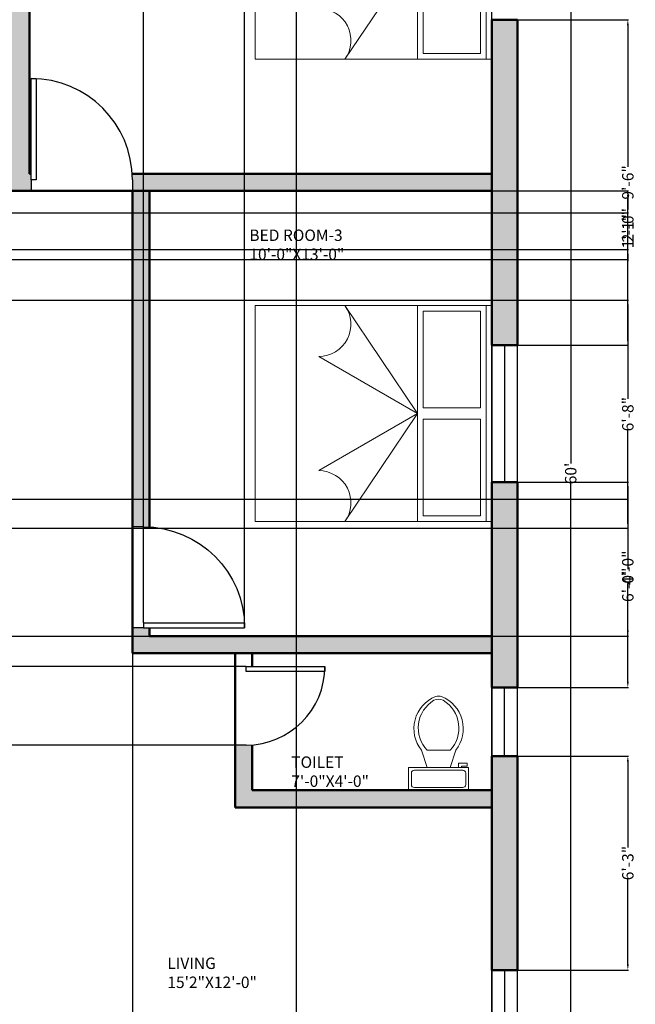
# Model space of a CAD drawing. Units: inches. Extents: x 2430 to 2930, y 1715 to 2575.
# Tile 3 of 4: x 2711 to 2927, y 1933 to 2278. Entities that reach past the tile are written whole.
import ezdxf

# ---------------------------------------------------------------- set-up
doc = ezdxf.new("R2010")
doc.units = ezdxf.units.IN
for name, color, linetype, lineweight in [('A-ANNO-DIMS', 2, 'Continuous', 18), ('A-AREA-IDEN', 130, 'Continuous', 18), ('A-FLOR-FIXT', 200, 'Continuous', 18), ('A-FURN', 200, 'Continuous', 18), ('A-WALL', 7, 'Continuous', 50), ('A-WALL-PATT', 251, 'Continuous', 13), ('DOOR', 224, 'Continuous', 25), ('win', 170, 'Continuous', 25)]:
    doc.layers.add(name, color=color, linetype=linetype, lineweight=lineweight)
doc.styles.get("Standard").update_dxf_attribs({"font": 'arial.ttf', "height": 4})
doc.dimstyles.get("Standard").update_dxf_attribs({"dimtxt": 4, "dimasz": 2, "dimexe": 0.18, "dimexo": 0.0625, "dimgap": 0.09, "dimtad": 0, "dimzin": 0, "dimdsep": 46, "dimlunit": 3, "dimtxsty": 'Standard', "dimcen": 0.09, "dimadec": 0, "dimazin": 0, "dimtfac": 1, "dimtofl": 0, "dimtmove": 0, "dimatfit": 3, "dimfxl": 1, "dimtolj": 1, "dimtzin": 0, "dimarcsym": 0})

# ---------------------------------------------------------------- blocks, each defined once
blk = doc.blocks.new('*U4')
for p, q in [((0, 0), (0, -100)), ((700, 0), (700, -100))]:
    blk.add_line(p, q)
blk.add_lwpolyline([(0, 0), (0, 700), (43.75, 700), (43.75, 0)], close=True)
blk.add_arc((0, 0), 700, 0, 90)
blk = doc.blocks.new('*U7')
for p, q in [((0, 0), (0, -100)), ((900, 0), (900, -100))]:
    blk.add_line(p, q)
blk.add_lwpolyline([(0, 0), (0, 900), (43.75, 900), (43.75, 0)], close=True)
blk.add_arc((0, 0), 900, 0, 90)
blk = doc.blocks.new('*U9')
for p, q in [((241.3, -152.4), (241.3, -50.8)), ((-254, -215.9), (-203.2, -215.9)), ((-254, -241.3), (-254, -215.9)), ((-177.8, -241.3), (-254, -241.3)), ((-203.2, -215.9), (-203.2, -203.2)), ((-177.8, -203.2), (-177.8, -241.3)), ((-101.6, -203.2), (-152.4, -355.6)), ((101.6, -203.2), (152.4, -355.6)), ((101.6, -355.6), (-101.6, -355.6))]:
    blk.add_line(p, q)
blk.add_lwpolyline([(266.7, -203.2), (266.7, 0), (-266.7, 0), (-266.7, -203.2)], close=True)
for points in [[(-241.3, -50.8), (-241.3, -152.4)], [(215.9, -25.4), (-215.9, -25.4)], [(-215.9, -177.8), (215.9, -177.8)]]:
    blk.add_lwpolyline(points)
for centre, radius, start, end in [((-219.1, -47.6), 22.5, 81.8699, 188.1301), ((219.1, -47.6), 22.5, 351.8699, 98.1301), ((-219.1, -155.6), 22.5, 171.8699, 278.1301), ((219.1, -155.6), 22.5, 261.8699, 8.1301), ((89.4, -548.1), 309.1, 141.46911, 247.97143), ((106.7, -554.2), 287.8, 136.36773, 238.94682), ((-89.4, -548.1), 309.1, 292.02843, 38.53071), ((-106.7, -554.2), 287.8, 301.05301, 43.63209), ((0, -708.1), 101.6, 245.73182, 294.26817), ((0, -736.6), 101.6, 254.86053, 285.13947)]:
    blk.add_arc(centre, radius, start, end)
blk = doc.blocks.new('NEW BED')
for p, q in [((-75.7, 82.92), (0, 82.92)), ((-75.7, 0), (-75.7, 82.92)), ((0, 82.92), (0, 0)), ((-75.7, 80.92), (0, 80.92)), ((-73.7, 78.92), (-39.85, 78.92)), ((-73.7, 58.92), (-73.7, 78.92)), ((-39.85, 58.92), (-39.85, 78.92)), ((-35.85, 78.92), (-2, 78.92)), ((-35.85, 58.92), (-35.85, 78.92)), ((-2, 78.92), (-2, 58.92)), ((-73.7, 58.92), (-39.85, 58.92)), ((-35.85, 58.92), (-2, 58.92)), ((-75.7, 56.92), (0, 56.92)), ((-37.85, 56.92), (-75.7, 31.45)), ((-37.85, 56.92), (-57.85, 22.27)), ((-37.85, 56.92), (0, 31.45)), ((-37.85, 56.92), (-17.84, 22.27)), ((0, 0), (-75.7, 0))]:
    blk.add_line(p, q)
for centre, start, end in [((-69.14, 22.27), 0, 125.5497), ((-6.56, 22.27), 54.4503, 180)]:
    blk.add_arc(centre, 11.28, start, end)
blk = doc.blocks.new('*D12')
at = {"layer": 'A-ANNO-DIMS', "color": 0, "lineweight": -2, "transparency": 16777216}
for p, q in [((2885.68, 2479.45), (2904.48, 2479.45)), ((2904.3, 2477.45), (2904.3, 2122.95)), ((2904.3, 1761.45), (2904.3, 2115.96)), ((2885.68, 1759.45), (2904.48, 1759.45))]:
    blk.add_line(p, q, dxfattribs=at)
at = {"layer": 'A-ANNO-DIMS', "color": 0, "transparency": 16777216}
for points in [[(2903.96, 2477.45), (2904.63, 2477.45), (2904.3, 2479.45)], [(2903.96, 1761.45), (2904.63, 1761.45), (2904.3, 1759.45)]]:
    blk.add_solid(points, dxfattribs=at)
at = {"layer": 'Defpoints', "color": 0, "transparency": 16777216}
for p in [(2885.62, 2479.45), (2885.62, 1759.45), (2904.3, 1759.45)]:
    blk.add_point(p, dxfattribs=at)
at = {"layer": 'A-ANNO-DIMS', "color": 0, "transparency": 16777216, "insert": (2904.3, 2119.45), "char_height": 4, "attachment_point": 5, "rotation": 90}
blk.add_mtext("\\A1;60'", dxfattribs=at)
blk = doc.blocks.new('WIN-48IN')
blk.add_line((0, 4.5), (48, 4.5))
blk.add_lwpolyline([(0, 9), (48, 9), (48, 0), (0, 0)], close=True)
blk = doc.blocks.new('WIN-24IN')
blk.add_line((24, 4.5), (0, 4.5))
blk.add_lwpolyline([(0, 9), (24, 9), (24, 0), (0, 0)], close=True)
blk = doc.blocks.new('*D25')
at = {"layer": 'A-ANNO-DIMS', "color": 0, "lineweight": -2, "transparency": 16777216}
for p, q in [((2754.56, 2067.12), (2754.56, 2569.33)), ((2756.56, 2569.15), (2760.62, 2569.15)), ((2787.99, 2569.15), (2783.93, 2569.15)), ((2789.99, 2067.12), (2789.99, 2569.33))]:
    blk.add_line(p, q, dxfattribs=at)
at = {"layer": 'A-ANNO-DIMS', "color": 0, "transparency": 16777216}
for points in [[(2756.56, 2569.49), (2756.56, 2568.82), (2754.56, 2569.15)], [(2787.99, 2569.49), (2787.99, 2568.82), (2789.99, 2569.15)]]:
    blk.add_solid(points, dxfattribs=at)
at = {"layer": 'Defpoints', "color": 0, "transparency": 16777216}
for p in [(2789.99, 2569.15), (2754.56, 2067.05), (2789.99, 2067.05)]:
    blk.add_point(p, dxfattribs=at)
at = {"layer": 'A-ANNO-DIMS', "color": 0, "transparency": 16777216, "insert": (2772.27, 2569.15), "char_height": 4, "attachment_point": 5}
blk.add_mtext('\\A1;2\'-11 1/2"', dxfattribs=at)
blk = doc.blocks.new('*D26')
at = {"layer": 'A-ANNO-DIMS', "color": 0, "lineweight": -2, "transparency": 16777216}
for p, q in [((2786.56, 2051.85), (2435.74, 2051.85)), ((2435.92, 2049.85), (2435.92, 2048.17)), ((2435.92, 2026.29), (2435.92, 2027.97)), ((2786.56, 2024.29), (2435.74, 2024.29))]:
    blk.add_line(p, q, dxfattribs=at)
at = {"layer": 'A-ANNO-DIMS', "color": 0, "transparency": 16777216}
for points in [[(2435.59, 2049.85), (2436.25, 2049.85), (2435.92, 2051.85)], [(2435.59, 2026.29), (2436.25, 2026.29), (2435.92, 2024.29)]]:
    blk.add_solid(points, dxfattribs=at)
at = {"layer": 'Defpoints', "color": 0, "transparency": 16777216}
for p in [(2435.92, 2051.85), (2786.62, 2051.85), (2786.62, 2024.29)]:
    blk.add_point(p, dxfattribs=at)
at = {"layer": 'A-ANNO-DIMS', "color": 0, "transparency": 16777216, "insert": (2435.92, 2038.07), "char_height": 4, "attachment_point": 5, "rotation": 90}
blk.add_mtext('\\A1;2\'-3 1/2"', dxfattribs=at)
blk = doc.blocks.new('*D35')
at = {"layer": 'A-ANNO-DIMS', "color": 0, "lineweight": -2, "transparency": 16777216}
for p, q in [((2885.68, 2278.45), (2924.5, 2278.45)), ((2924.32, 2276.45), (2924.32, 2226.86)), ((2924.32, 2166.45), (2924.32, 2216.05)), ((2885.68, 2164.45), (2924.5, 2164.45))]:
    blk.add_line(p, q, dxfattribs=at)
at = {"layer": 'A-ANNO-DIMS', "color": 0, "transparency": 16777216}
for points in [[(2923.99, 2276.45), (2924.65, 2276.45), (2924.32, 2278.45)], [(2923.99, 2166.45), (2924.65, 2166.45), (2924.32, 2164.45)]]:
    blk.add_solid(points, dxfattribs=at)
at = {"layer": 'Defpoints', "color": 0, "transparency": 16777216}
for p in [(2885.62, 2278.45), (2885.62, 2164.45), (2924.32, 2164.45)]:
    blk.add_point(p, dxfattribs=at)
at = {"layer": 'A-ANNO-DIMS', "color": 0, "transparency": 16777216, "insert": (2924.32, 2221.45), "char_height": 4, "attachment_point": 5, "rotation": 90}
blk.add_mtext('\\A1;9\'-6"', dxfattribs=at)
blk = doc.blocks.new('*D36')
at = {"layer": 'A-ANNO-DIMS', "color": 0, "lineweight": -2, "transparency": 16777216}
for p, q in [((2885.68, 2116.45), (2924.5, 2116.45)), ((2924.32, 2114.45), (2924.32, 2085.87)), ((2924.32, 2046.45), (2924.32, 2075.04)), ((2885.68, 2044.45), (2924.5, 2044.45))]:
    blk.add_line(p, q, dxfattribs=at)
at = {"layer": 'A-ANNO-DIMS', "color": 0, "transparency": 16777216}
for points in [[(2923.99, 2114.45), (2924.65, 2114.45), (2924.32, 2116.45)], [(2923.99, 2046.45), (2924.65, 2046.45), (2924.32, 2044.45)]]:
    blk.add_solid(points, dxfattribs=at)
at = {"layer": 'Defpoints', "color": 0, "transparency": 16777216}
for p in [(2885.62, 2116.45), (2885.62, 2044.45), (2924.32, 2044.45)]:
    blk.add_point(p, dxfattribs=at)
at = {"layer": 'A-ANNO-DIMS', "color": 0, "transparency": 16777216, "insert": (2924.32, 2080.45), "char_height": 4, "attachment_point": 5, "rotation": 90}
blk.add_mtext('\\A1;6\'-0"', dxfattribs=at)
blk = doc.blocks.new('*D37')
at = {"layer": 'A-ANNO-DIMS', "color": 0, "lineweight": -2, "transparency": 16777216}
for p, q in [((2885.68, 2020.45), (2924.5, 2020.45)), ((2924.32, 2018.45), (2924.32, 1988.37)), ((2924.32, 1947.45), (2924.32, 1977.54)), ((2885.68, 1945.45), (2924.5, 1945.45))]:
    blk.add_line(p, q, dxfattribs=at)
at = {"layer": 'A-ANNO-DIMS', "color": 0, "transparency": 16777216}
for points in [[(2923.99, 2018.45), (2924.65, 2018.45), (2924.32, 2020.45)], [(2923.99, 1947.45), (2924.65, 1947.45), (2924.32, 1945.45)]]:
    blk.add_solid(points, dxfattribs=at)
at = {"layer": 'Defpoints', "color": 0, "transparency": 16777216}
for p in [(2885.62, 2020.45), (2885.62, 1945.45), (2924.32, 1945.45)]:
    blk.add_point(p, dxfattribs=at)
at = {"layer": 'A-ANNO-DIMS', "color": 0, "transparency": 16777216, "insert": (2924.32, 1982.95), "char_height": 4, "attachment_point": 5, "rotation": 90}
blk.add_mtext('\\A1;6\'-3"', dxfattribs=at)
blk = doc.blocks.new('*D39')
at = {"layer": 'A-ANNO-DIMS', "color": 0, "lineweight": -2, "transparency": 16777216}
for p, q in [((2808.12, 1840.52), (2808.12, 2569.33)), ((2810.12, 2569.15), (2832.3, 2569.15)), ((2874.62, 2569.15), (2852.44, 2569.15)), ((2876.62, 1840.52), (2876.62, 2569.33))]:
    blk.add_line(p, q, dxfattribs=at)
at = {"layer": 'A-ANNO-DIMS', "color": 0, "transparency": 16777216}
for points in [[(2810.12, 2569.49), (2810.12, 2568.82), (2808.12, 2569.15)], [(2874.62, 2569.49), (2874.62, 2568.82), (2876.62, 2569.15)]]:
    blk.add_solid(points, dxfattribs=at)
at = {"layer": 'Defpoints', "color": 0, "transparency": 16777216}
for p in [(2876.62, 2569.15), (2808.12, 1840.45), (2876.62, 1840.45)]:
    blk.add_point(p, dxfattribs=at)
at = {"layer": 'A-ANNO-DIMS', "color": 0, "transparency": 16777216, "insert": (2842.37, 2569.15), "char_height": 4, "attachment_point": 5}
blk.add_mtext('\\A1;5\'-8 1/2"', dxfattribs=at)
blk = doc.blocks.new('*D40')
at = {"layer": 'A-ANNO-DIMS', "color": 0, "lineweight": -2, "transparency": 16777216}
for p, q in [((2630.68, 2180.15), (2924.5, 2180.15)), ((2924.32, 2178.15), (2924.32, 2145.66)), ((2924.32, 2102.32), (2924.32, 2134.82)), ((2630.68, 2100.32), (2924.5, 2100.32))]:
    blk.add_line(p, q, dxfattribs=at)
at = {"layer": 'A-ANNO-DIMS', "color": 0, "transparency": 16777216}
for points in [[(2923.99, 2178.15), (2924.65, 2178.15), (2924.32, 2180.15)], [(2923.99, 2102.32), (2924.65, 2102.32), (2924.32, 2100.32)]]:
    blk.add_solid(points, dxfattribs=at)
at = {"layer": 'Defpoints', "color": 0, "transparency": 16777216}
for p in [(2630.62, 2180.15), (2924.32, 2180.15), (2630.62, 2100.32)]:
    blk.add_point(p, dxfattribs=at)
at = {"layer": 'A-ANNO-DIMS', "color": 0, "transparency": 16777216, "insert": (2924.32, 2140.24), "char_height": 4, "attachment_point": 5, "rotation": 90}
blk.add_mtext('\\A1;6\'-8"', dxfattribs=at)
blk = doc.blocks.new('*D41')
at = {"layer": 'A-ANNO-DIMS', "color": 0, "lineweight": -2, "transparency": 16777216}
for p, q in [((2693.62, 2062.39), (2693.62, 1720.57)), ((2750.62, 2056.39), (2750.62, 1720.57)), ((2695.62, 1720.75), (2716.63, 1720.75)), ((2748.62, 1720.75), (2727.61, 1720.75))]:
    blk.add_line(p, q, dxfattribs=at)
at = {"layer": 'A-ANNO-DIMS', "color": 0, "transparency": 16777216}
for points in [[(2695.62, 1721.09), (2695.62, 1720.42), (2693.62, 1720.75)], [(2748.62, 1721.09), (2748.62, 1720.42), (2750.62, 1720.75)]]:
    blk.add_solid(points, dxfattribs=at)
at = {"layer": 'Defpoints', "color": 0, "transparency": 16777216}
for p in [(2693.62, 2062.45), (2750.62, 2056.45), (2750.62, 1720.75)]:
    blk.add_point(p, dxfattribs=at)
at = {"layer": 'A-ANNO-DIMS', "color": 0, "transparency": 16777216, "insert": (2722.12, 1720.75), "char_height": 4, "attachment_point": 5}
blk.add_mtext('\\A1;4\'-9"', dxfattribs=at)
blk = doc.blocks.new('*D50')
at = {"layer": 'A-ANNO-DIMS', "color": 0, "lineweight": -2, "transparency": 16777216}
for p, q in [((2536.91, 2110.42), (2924.5, 2110.42)), ((2924.32, 2108.42), (2924.32, 2091.92)), ((2924.32, 2064.45), (2924.32, 2080.95)), ((2534.68, 2062.45), (2924.5, 2062.45))]:
    blk.add_line(p, q, dxfattribs=at)
at = {"layer": 'A-ANNO-DIMS', "color": 0, "transparency": 16777216}
for points in [[(2923.99, 2108.42), (2924.65, 2108.42), (2924.32, 2110.42)], [(2923.99, 2064.45), (2924.65, 2064.45), (2924.32, 2062.45)]]:
    blk.add_solid(points, dxfattribs=at)
at = {"layer": 'Defpoints', "color": 0, "transparency": 16777216}
for p in [(2536.85, 2110.42), (2534.62, 2062.45), (2924.32, 2062.45)]:
    blk.add_point(p, dxfattribs=at)
at = {"layer": 'A-ANNO-DIMS', "color": 0, "transparency": 16777216, "insert": (2924.32, 2086.44), "char_height": 4, "attachment_point": 5, "rotation": 90}
blk.add_mtext('\\A1;4\'-0"', dxfattribs=at)
blk = doc.blocks.new('*D52')
at = {"layer": 'A-ANNO-DIMS', "color": 0, "lineweight": -2, "transparency": 16777216}
for p, q in [((2924.32, 2212.78), (2924.32, 2214.78)), ((2608.57, 2210.78), (2924.5, 2210.78)), ((2613.81, 2197.89), (2924.5, 2197.89)), ((2924.32, 2195.89), (2924.32, 2193.89))]:
    blk.add_line(p, q, dxfattribs=at)
at = {"layer": 'A-ANNO-DIMS', "color": 0, "transparency": 16777216}
for points in [[(2923.99, 2212.78), (2924.65, 2212.78), (2924.32, 2210.78)], [(2923.99, 2195.89), (2924.65, 2195.89), (2924.32, 2197.89)]]:
    blk.add_solid(points, dxfattribs=at)
at = {"layer": 'Defpoints', "color": 0, "transparency": 16777216}
for p in [(2608.51, 2210.78), (2924.32, 2210.78), (2613.75, 2197.89)]:
    blk.add_point(p, dxfattribs=at)
at = {"layer": 'A-ANNO-DIMS', "color": 0, "transparency": 16777216, "insert": (2924.32, 2204.34), "char_height": 4, "attachment_point": 5, "rotation": 90}
blk.add_mtext('\\A1;1\'-1"', dxfattribs=at)
blk = doc.blocks.new('*D54')
at = {"layer": 'A-ANNO-DIMS', "color": 0, "lineweight": -2, "transparency": 16777216}
for p, q in [((2624.68, 2218.45), (2924.5, 2218.45)), ((2924.32, 2216.45), (2924.32, 2211.89)), ((2924.32, 2196.45), (2924.32, 2201.01)), ((2624.68, 2194.45), (2924.5, 2194.45))]:
    blk.add_line(p, q, dxfattribs=at)
at = {"layer": 'A-ANNO-DIMS', "color": 0, "transparency": 16777216}
for points in [[(2923.99, 2216.45), (2924.65, 2216.45), (2924.32, 2218.45)], [(2923.99, 2196.45), (2924.65, 2196.45), (2924.32, 2194.45)]]:
    blk.add_solid(points, dxfattribs=at)
at = {"layer": 'Defpoints', "color": 0, "transparency": 16777216}
for p in [(2624.62, 2218.45), (2924.32, 2218.45), (2624.62, 2194.45)]:
    blk.add_point(p, dxfattribs=at)
at = {"layer": 'A-ANNO-DIMS', "color": 0, "transparency": 16777216, "insert": (2924.32, 2206.45), "char_height": 4, "attachment_point": 5, "rotation": 90}
blk.add_mtext('\\A1;2\'-0"', dxfattribs=at)

msp = doc.modelspace()

# ---------------------------------------------------------------- hatches: boundary and pattern name
at = {"layer": 'A-WALL-PATT'}
h = msp.add_hatch(color=256, dxfattribs=at)
h.dxf.hatch_style = 1
h.paths.add_polyline_path([(2714.621, 2380.453), (2707.621, 2380.453), (2707.621, 2224.453), (2705.621, 2224.453), (2705.621, 2222.39), (2705.621, 2218.453), (2715.188, 2218.453), (2715.188, 2222.39), (2715.188, 2224.453), (2714.621, 2224.453)])
h.paths.add_polyline_path([(2756.969, 2384.39, -0.0145648), (2757.029, 2386.453), (2654.378, 2386.453, -0.0145648), (2654.438, 2384.39), (2654.438, 2380.453), (2756.969, 2380.453)])
h = msp.add_hatch(color=256, dxfattribs=at)
h.dxf.hatch_style = 1
h.paths.add_polyline_path([(2885.621, 2116.453), (2876.621, 2116.453), (2876.621, 2044.453), (2885.621, 2044.453)])
h.paths.add_polyline_path([(2876.621, 2062.453), (2756.621, 2062.453), (2756.621, 2065.333), (2754.558, 2065.333), (2750.621, 2065.333), (2750.621, 2062.453), (2750.621, 2056.453), (2876.621, 2056.453)])
h.paths.add_polyline_path([(2885.621, 2278.453), (2876.621, 2278.453), (2876.621, 2164.453), (2885.621, 2164.453)])
h.paths.add_polyline_path([(2876.621, 2224.453), (2750.561, 2224.453, -0.0145648), (2750.621, 2222.39), (2750.621, 2218.453), (2876.621, 2218.453)])
h.paths.add_polyline_path([(2756.621, 2218.453), (2750.621, 2218.453), (2750.621, 2100.766), (2754.558, 2100.766, -0.0145648), (2756.621, 2100.706)])
h.paths.add_polyline_path([(2630.621, 2100.325), (2624.621, 2100.325), (2624.621, 2062.453), (2534.621, 2062.453), (2534.621, 2053.453), (2646.072, 2053.453), (2646.072, 2057.39, -0.0403846), (2646.482, 2062.453), (2630.621, 2062.453)])
h.paths.add_polyline_path([(2534.621, 2140.453), (2525.621, 2140.453), (2525.621, 2038.453), (2534.621, 2038.453)])
h.paths.add_polyline_path([(2670.188, 2222.39, -0.0145648), (2670.248, 2224.453), (2534.621, 2224.453), (2534.621, 2218.453), (2670.188, 2218.453)])
h.paths.add_polyline_path([(2630.621, 2218.453), (2624.621, 2218.453), (2624.621, 2180.154), (2630.621, 2180.154)])
h.paths.add_polyline_path([(2534.621, 2278.453), (2525.621, 2278.453), (2525.621, 2188.453), (2534.621, 2188.453)])
h = msp.add_hatch(color=256, dxfattribs=at)
h.dxf.hatch_style = 1
h.paths.add_polyline_path([(2885.621, 1897.453), (2876.621, 1897.453), (2876.621, 1769.453), (2682.621, 1769.453), (2682.621, 1759.453), (2885.621, 1759.453)])
h.paths.add_polyline_path([(2885.621, 2020.453), (2876.621, 2020.453), (2876.621, 1945.453), (2885.621, 1945.453)])
h.paths.add_polyline_path([(2876.621, 1840.453), (2808.121, 1840.453), (2808.121, 1831.453), (2876.621, 1831.453)], flags=17)
h.paths.add_polyline_path([(2760.121, 1840.453), (2691.621, 1840.453), (2691.621, 1849.896), (2686.558, 1849.896), (2682.621, 1849.896), (2682.621, 1831.453), (2760.121, 1831.453)], flags=17)
h.paths.add_polyline_path([(2691.621, 1915.889), (2682.621, 1915.889), (2682.621, 1889.266), (2686.558, 1889.266, -0.0322505), (2691.621, 1888.939)])
h.paths.add_polyline_path([(2691.621, 2056.453), (2693.621, 2056.453), (2693.621, 2062.453), (2682.621, 2062.453), (2677.568, 2062.453), (2677.568, 2057.39), (2677.568, 2053.453), (2682.621, 2053.453), (2682.621, 1975.453), (2673.244, 1975.453), (2673.244, 1970.39), (2673.244, 1966.453), (2682.621, 1966.453), (2682.621, 1963.889), (2691.621, 1963.889)])
h.paths.add_polyline_path([(2641.748, 1970.39, -0.0403846), (2642.158, 1975.453), (2534.621, 1975.453), (2534.621, 1966.453), (2641.748, 1966.453)])
h.paths.add_polyline_path([(2534.621, 1990.453), (2525.621, 1990.453), (2525.621, 1759.453), (2534.621, 1759.453)])
h = msp.add_hatch(color=256, dxfattribs=at)
h.dxf.hatch_style = 1
h.paths.add_polyline_path([(2876.621, 2008.453), (2792.621, 2008.453), (2792.621, 2024.365, -0.018734), (2790.558, 2024.288), (2786.621, 2024.288), (2786.621, 2002.453), (2876.621, 2002.453)])

# ---------------------------------------------------------------- linework, layer by layer
at = {"layer": 'A-WALL'}
for p, q in [((2714.621, 2224.453), (2714.621, 2380.453)), ((2876.621, 2278.453), (2885.621, 2278.453)), ((2876.621, 2278.453), (2876.621, 2164.453)), ((2714.621, 2224.453), (2715.188, 2224.453)), ((2750.561, 2224.453), (2876.621, 2224.453)), ((2534.621, 2218.453), (2876.621, 2218.453)), ((2750.621, 2062.453), (2750.621, 2218.453)), ((2756.621, 2100.706), (2756.621, 2218.453)), ((2876.621, 2164.453), (2885.621, 2164.453)), ((2876.621, 2116.453), (2885.621, 2116.453)), ((2876.621, 2116.453), (2876.621, 2044.453)), ((2756.621, 2062.453), (2756.621, 2065.333)), ((2750.621, 2056.453), (2750.621, 2062.453)), ((2756.621, 2062.453), (2876.621, 2062.453)), ((2750.621, 2056.453), (2876.621, 2056.453)), ((2786.621, 2056.453), (2786.621, 2002.453)), ((2792.621, 2056.453), (2792.621, 2051.847)), ((2876.621, 2044.453), (2885.621, 2044.453)), ((2792.621, 2024.365), (2792.621, 2008.453)), ((2876.621, 2020.453), (2885.621, 2020.453)), ((2876.621, 2020.453), (2876.621, 1945.453)), ((2792.621, 2008.453), (2876.621, 2008.453)), ((2786.621, 2002.453), (2876.621, 2002.453)), ((2876.621, 1945.453), (2885.621, 1945.453))]:
    msp.add_line(p, q, dxfattribs=at)
for points in [[(2885.621, 2278.453), (2885.621, 2164.453)], [(2885.621, 2116.453), (2885.621, 2044.453)], [(2885.621, 2020.453), (2885.621, 1945.453)]]:
    msp.add_lwpolyline(points, dxfattribs=at)

# ---------------------------------------------------------------- block references
at = {"layer": 'A-FLOR-FIXT', "xscale": 0.0393700787401575, "yscale": 0.0393700787401575, "zscale": 0.0393700787401575, "rotation": 180}
msp.add_blockref('*U9', (2857.979, 2008.453), dxfattribs=at)
at = {"layer": 'A-FURN', "xscale": -1, "rotation": 270}
for p in [(2793.7, 2340.302), (2793.7, 2178.302)]:
    msp.add_blockref('NEW BED', p, dxfattribs=at)
at = {"layer": 'DOOR', "xscale": 0.0393700787401575, "yscale": 0.0393700787401575, "zscale": 0.0393700787401575}
msp.add_blockref('*U7', (2715.188, 2222.39), dxfattribs=at)
at = {"layer": 'DOOR', "yscale": 0.0393700787401575, "zscale": 0.0393700787401575, "rotation": 270}
for name, p, xscale in [('*U7', (2754.558, 2065.333), -0.0393700787401575), ('*U4', (2790.558, 2051.847), 0.0393700787401575)]:
    msp.add_blockref(name, p, dxfattribs=dict(at, xscale=xscale))
at = {"layer": 'win', "extrusion": (0, 0, -1), "zscale": -1}
for name, p, rotation in [('WIN-48IN', (-2885.621, 2164.453), 270.0000000000006), ('WIN-24IN', (-2885.621, 2044.453), 270.0000000000013), ('WIN-48IN', (-2885.621, 1945.453), 270.0000000000005)]:
    msp.add_blockref(name, p, dxfattribs=dict(at, rotation=rotation))

# ---------------------------------------------------------------- texts
at = {"layer": 'A-AREA-IDEN', "char_height": 4, "attachment_point": 1}
for s, width, insert in [('BED ROOM-3\\P10\'-0"X13\'-0"', 55.10797, (2791.635, 2204.917)), ('TOILET\\P7\'-0"X4\'-0"', 27.45852, (2806.329, 2020.305)), ('LIVING\\P15\'2"X12\'-0"', 48.99066, (2762.89, 1949.834))]:
    msp.add_mtext_dynamic_manual_height_columns(s, width=width, gutter_width=20, heights=[0], dxfattribs=dict(at, insert=insert))

# ---------------------------------------------------------------- dimensions: what is measured, and where the dimension line sits
at = {"layer": 'A-ANNO-DIMS'}
for base, p1, p2, picture, middle in [((2789.991, 2569.153), (2754.558, 2067.055), (2789.991, 2067.055), '*D25', (2772.275, 2569.153)), ((2876.621, 2569.153), (2808.121, 1840.453), (2876.621, 1840.453), '*D39', (2842.371, 2569.153)), ((2750.621, 1720.753), (2693.621, 2062.453), (2750.621, 2056.453), '*D41', (2722.121, 1720.753))]:
    dim = msp.add_linear_dim(base=base, p1=p1, p2=p2, dimstyle='Standard', override={"dimdec": 1, "dimlfac": 1, "dimrnd": 0, "dimzin": 1, "dimdsep": 46, "dimlunit": 4, "dimfrac": 2}, dxfattribs=at)
    dim.commit()
    dim.dimension.update_dxf_attribs({"geometry": picture, "text_midpoint": middle})
for base, p1, p2, override, picture, middle in [((2904.296, 1759.453), (2885.621, 2479.453), (2885.621, 1759.453), {"dimclrd": 0, "dimclre": 0, "dimclrt": 0}, '*D12', (2904.296, 2119.453)), ((2924.321, 2164.453), (2885.621, 2278.453), (2885.621, 2164.453), {"dimdec": 1, "dimlfac": 1, "dimrnd": 0, "dimzin": 1, "dimdsep": 46, "dimlunit": 4, "dimfrac": 2}, '*D35', (2924.321, 2221.453)), ((2924.321, 2218.453), (2624.621, 2194.453), (2624.621, 2218.453), {"dimdec": 1, "dimlfac": 1, "dimrnd": 0, "dimzin": 1, "dimdsep": 46, "dimlunit": 4, "dimfrac": 2}, '*D54', (2924.321, 2206.453)), ((2924.321, 2210.778), (2613.749, 2197.895), (2608.51, 2210.778), {"dimdec": 1, "dimlfac": 1, "dimrnd": 0, "dimzin": 1, "dimdsep": 46, "dimlunit": 4, "dimfrac": 2}, '*D52', (2924.321, 2204.336)), ((2924.321, 2180.154), (2630.621, 2100.325), (2630.621, 2180.154), {"dimdec": 1, "dimlfac": 1, "dimrnd": 0, "dimzin": 1, "dimdsep": 46, "dimlunit": 4, "dimfrac": 2}, '*D40', (2924.321, 2140.239)), ((2924.321, 2044.453), (2885.621, 2116.453), (2885.621, 2044.453), {"dimdec": 1, "dimlfac": 1, "dimrnd": 0, "dimzin": 1, "dimdsep": 46, "dimlunit": 4, "dimfrac": 2}, '*D36', (2924.321, 2080.453)), ((2924.321, 2062.453), (2536.852, 2110.422), (2534.621, 2062.453), {"dimdec": 1, "dimlfac": 1, "dimrnd": 0, "dimzin": 1, "dimdsep": 46, "dimlunit": 4, "dimfrac": 2}, '*D50', (2924.321, 2086.438)), ((2435.921, 2051.847), (2786.621, 2024.288), (2786.621, 2051.847), {"dimdec": 1, "dimlfac": 1, "dimrnd": 0, "dimzin": 1, "dimdsep": 46, "dimlunit": 4, "dimfrac": 2}, '*D26', (2435.921, 2038.067)), ((2924.321, 1945.453), (2885.621, 2020.453), (2885.621, 1945.453), {"dimdec": 1, "dimlfac": 1, "dimrnd": 0, "dimzin": 1, "dimdsep": 46, "dimlunit": 4, "dimfrac": 2}, '*D37', (2924.321, 1982.953))]:
    dim = msp.add_linear_dim(base=base, p1=p1, p2=p2, angle=90, dimstyle='Standard', override=override, dxfattribs=at)
    dim.commit()
    dim.dimension.update_dxf_attribs({"geometry": picture, "text_midpoint": middle})

doc.saveas('drawing.dxf')
